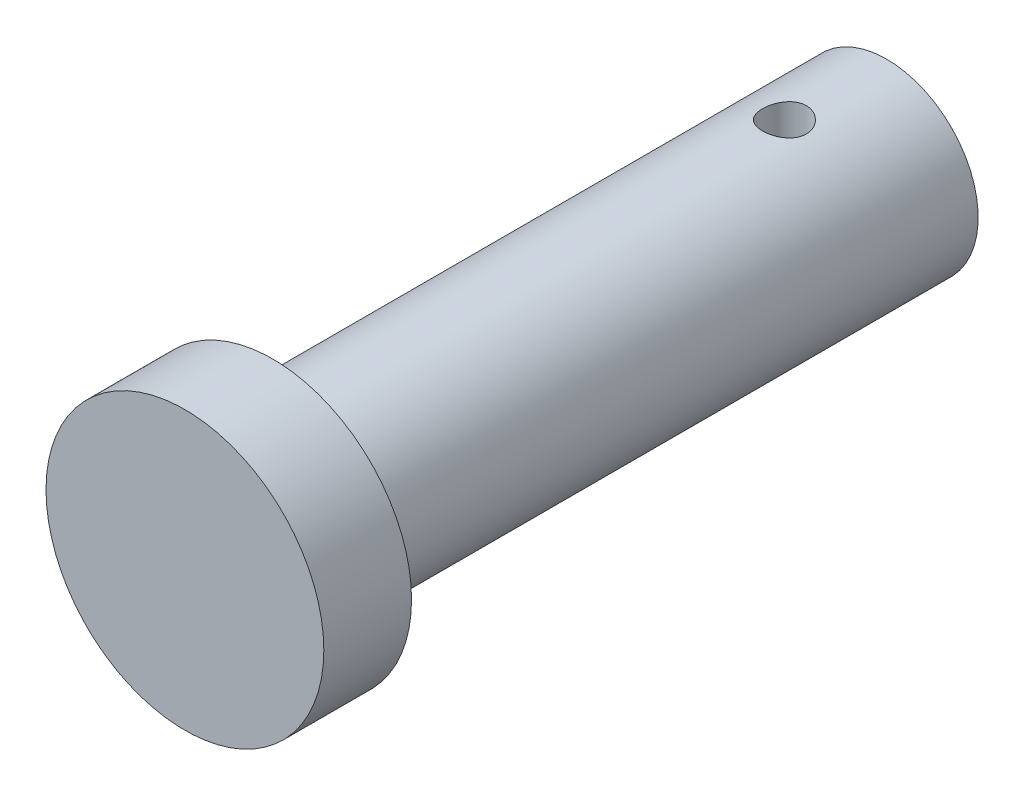
SolidWorks part; units mm, degrees
material "Plain Carbon Steel"
ref_plane "Front Plane" through (0, 0, 0) normal (0, 0, 1) x (1, 0, 0)
ref_plane "Top Plane" through (0, 0, 0) normal (0, 1, 0) x (1, 0, 0)
ref_plane "Right Plane" through (0, 0, 0) normal (1, 0, 0) x (0, 0, -1)
sketch "Head Profile Ø38" plane through (0, 0, 0) normal (0, 0, 1) x (1, 0, 0)
  circle A0 centre (0, 0) radius 19
  dimension "D1" = 38
extrude "Head Ø38x12" add sketch "Head Profile Ø38" along normal blind 12
sketch "Shank Profile Ø25" plane through (0, 0, 0) normal (0, 0, -1) x (-1, 0, 0)
  circle A0 centre (0, 0) radius 12.5
  dimension "D1" = 25
extrude "Shank Ø25x84" add sketch "Shank Profile Ø25" along normal blind 84
sketch "Cross Hole Profile Ø6" plane through (0, 0, 0) normal (0, 1, 0) x (1, 0, 0)
  line L0 (0, 95.5684) -> (0, 70) construction
  line L1 (12.5, 84) -> (-12.5, 84) construction
  circle A0 centre (0, 70) radius 3
  dimension "D1" = 6
  dimension "D2" = 14
extrude "Cross Hole Ø6" cut sketch "Cross Hole Profile Ø6" against normal mid plane 84
